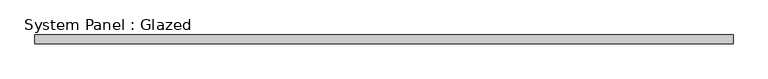
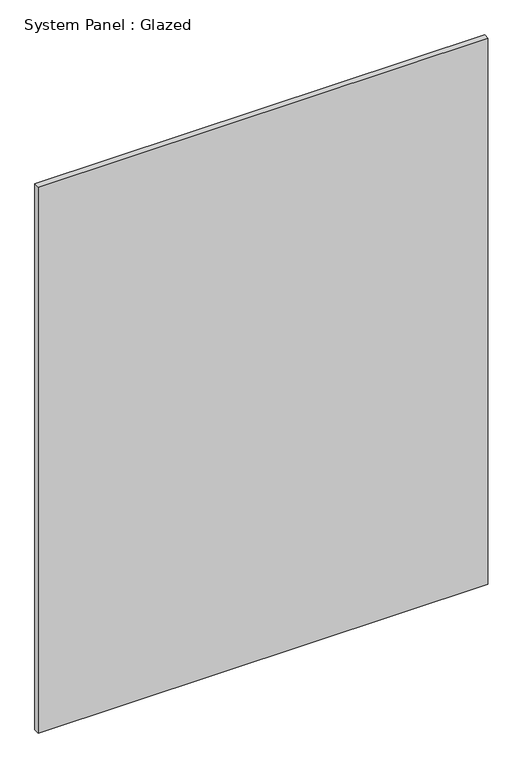
"""IFC4 building model written with IfcOpenShell, lengths in millimetres: plate geometry, System Panel : Glazed."""

from ifc_helpers import new_model, si_unit, origin, origin_with_axes, place, context, project, spatial, polyline, outline, extrude, source, transform, mapped, element, save


def system_panel_glazed_ffba6474(model_context):
    return source(origin(), model_context, "Body", "SweptSolid", [
        extrude(outline(polyline([(1019.175, 19.05), (-1019.175, 19.05), (-1019.175, 44.45), (1019.175, 44.45), (1019.175, 19.05)])), origin_with_axes(), (0.0, 0.0, 1.0), 2616.2),
    ])


if __name__ == "__main__":
    model = new_model("IFC4")
    model_context = context("Model", 3, world=origin())
    ifc_project = project(units=[si_unit("LENGTHUNIT", "METRE", prefix="MILLI")], contexts=[model_context])
    site = spatial("IfcSite", under=ifc_project)
    building = spatial("IfcBuilding", under=site)
    placement = place(None, origin())
    system_panel_glazed_shape = system_panel_glazed_ffba6474(model_context)
    element("IfcPlate", 1, ObjectType="System Panel : Glazed", at=placement, inside=building, context=model_context, shape_type="MappedRepresentation", body=[
        mapped(system_panel_glazed_shape, transform((0.0, 0.0, 0.0), x_axis=(1.0, 0.0, 0.0), y_axis=(0.0, 1.0, 0.0), z_axis=(0.0, 0.0, 1.0))),
    ])
    save(model, "model.ifc")

# Revit data of these elements
# Type "System Panel : Glazed"
#   Construction Type Id = "GSP4R"
#   Analytic Construction = "1/8 in Pilkington single glazing"
#   Visual Light Transmittance = 0.9
#   Solar Heat Gain Coefficient = 0.86
#   Heat Transfer Coefficient (U) = 1.18115 BTU/(h·ft²·°F)
# Element 1 (IfcPlate, "System Panel : Glazed")
#   Materials on its faces: "Glass"
# Materials
#   "Glass": class "Glass", colour RGB 0 128 192, transparency 0.75, Description = "Soda Lime Glass", Cost = 0
